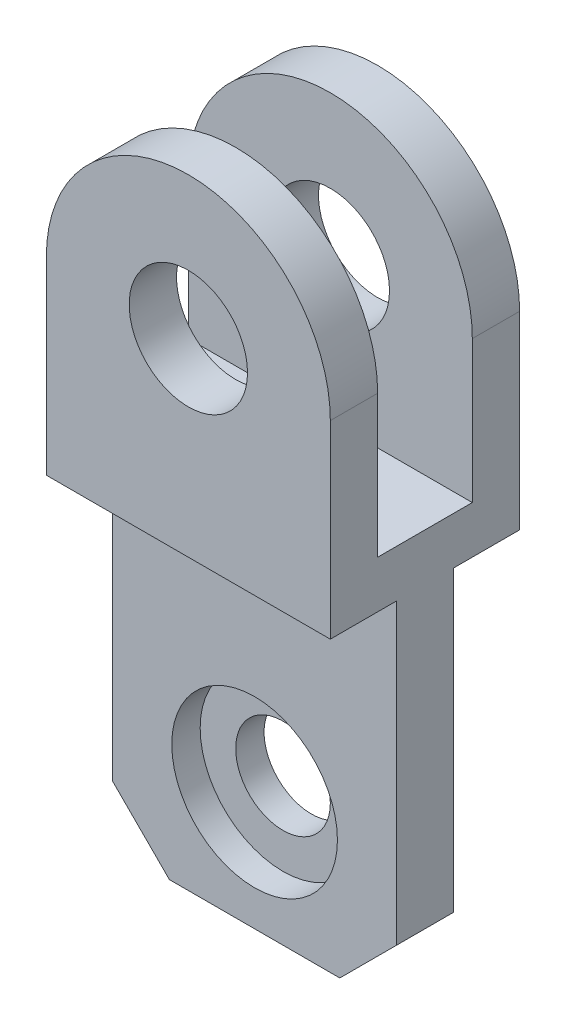
ISO-10303-21;
HEADER;
FILE_DESCRIPTION(('STEP AP214'),'2;1');
FILE_NAME('part.step','',(''),(''),'','','');
FILE_SCHEMA(('AUTOMOTIVE_DESIGN { 1 0 10303 214 1 1 1 1 }'));
ENDSEC;
DATA;
#1=APPLICATION_CONTEXT('core data for automotive mechanical design processes');
#2=APPLICATION_PROTOCOL_DEFINITION('international standard','automotive_design',2000,#1);
#3=PRODUCT_CONTEXT('',#1,'mechanical');
#4=PRODUCT('Part','Part','',(#3));
#5=PRODUCT_RELATED_PRODUCT_CATEGORY('part','',(#4));
#6=PRODUCT_DEFINITION_FORMATION('','',#4);
#7=PRODUCT_DEFINITION_CONTEXT('part definition',#1,'design');
#8=PRODUCT_DEFINITION('design','',#6,#7);
#9=PRODUCT_DEFINITION_SHAPE('','',#8);
#10=(LENGTH_UNIT() NAMED_UNIT(*) SI_UNIT(.MILLI.,.METRE.));
#11=(NAMED_UNIT(*) PLANE_ANGLE_UNIT() SI_UNIT($,.RADIAN.));
#12=(NAMED_UNIT(*) SI_UNIT($,.STERADIAN.) SOLID_ANGLE_UNIT());
#13=UNCERTAINTY_MEASURE_WITH_UNIT(LENGTH_MEASURE(1.E-05),#10,'distance_accuracy_value','');
#14=(GEOMETRIC_REPRESENTATION_CONTEXT(3) GLOBAL_UNCERTAINTY_ASSIGNED_CONTEXT((#13)) GLOBAL_UNIT_ASSIGNED_CONTEXT((#10,
#11,#12)) REPRESENTATION_CONTEXT('',''));
#15=CARTESIAN_POINT('',(0.,0.,0.));
#16=DIRECTION('',(0.,0.,1.));
#17=DIRECTION('',(1.,0.,0.));
#18=AXIS2_PLACEMENT_3D('',#15,#16,#17);
#19=CARTESIAN_POINT('',(-6.,0.,12.));
#20=DIRECTION('',(1.,0.,0.));
#21=DIRECTION('',(0.,0.,-1.));
#22=AXIS2_PLACEMENT_3D('',#19,#20,#21);
#23=PLANE('',#22);
#24=DIRECTION('',(0.,-1.,0.));
#25=VECTOR('',#24,1.);
#26=CARTESIAN_POINT('',(-6.,0.,0.));
#27=LINE('',#26,#25);
#28=CARTESIAN_POINT('',(-6.,0.,0.));
#29=VERTEX_POINT('',#28);
#30=CARTESIAN_POINT('',(-6.,-63.,0.));
#31=VERTEX_POINT('',#30);
#32=EDGE_CURVE('E126',#29,#31,#27,.T.);
#33=ORIENTED_EDGE('',*,*,#32,.T.);
#34=DIRECTION('',(0.,0.,-1.));
#35=VECTOR('',#34,1.);
#36=CARTESIAN_POINT('',(-6.,-63.,12.));
#37=LINE('',#36,#35);
#38=CARTESIAN_POINT('',(-6.,-63.,12.));
#39=VERTEX_POINT('',#38);
#40=EDGE_CURVE('E11',#39,#31,#37,.T.);
#41=ORIENTED_EDGE('',*,*,#40,.F.);
#42=DIRECTION('',(0.,-1.,0.));
#43=VECTOR('',#42,1.);
#44=CARTESIAN_POINT('',(-6.,0.,12.));
#45=LINE('',#44,#43);
#46=CARTESIAN_POINT('',(-6.,0.,12.));
#47=VERTEX_POINT('',#46);
#48=EDGE_CURVE('E107',#47,#39,#45,.T.);
#49=ORIENTED_EDGE('',*,*,#48,.F.);
#50=DIRECTION('',(0.,0.,1.));
#51=VECTOR('',#50,1.);
#52=CARTESIAN_POINT('',(-6.,0.,16.));
#53=LINE('',#52,#51);
#54=CARTESIAN_POINT('',(-6.,0.,26.));
#55=VERTEX_POINT('',#54);
#56=EDGE_CURVE('E91',#47,#55,#53,.T.);
#57=ORIENTED_EDGE('',*,*,#56,.T.);
#58=DIRECTION('',(0.,1.,0.));
#59=VECTOR('',#58,1.);
#60=CARTESIAN_POINT('',(-6.,0.,26.));
#61=LINE('',#60,#59);
#62=CARTESIAN_POINT('',(-6.,40.,26.));
#63=VERTEX_POINT('',#62);
#64=EDGE_CURVE('E235',#55,#63,#61,.T.);
#65=ORIENTED_EDGE('',*,*,#64,.T.);
#66=DIRECTION('',(0.,0.,-1.));
#67=VECTOR('',#66,1.);
#68=CARTESIAN_POINT('',(-6.,40.,26.));
#69=LINE('',#68,#67);
#70=CARTESIAN_POINT('',(-6.,40.,16.));
#71=VERTEX_POINT('',#70);
#72=EDGE_CURVE('E232',#63,#71,#69,.T.);
#73=ORIENTED_EDGE('',*,*,#72,.T.);
#74=DIRECTION('',(0.,1.,0.));
#75=VECTOR('',#74,1.);
#76=CARTESIAN_POINT('',(-6.,0.,16.));
#77=LINE('',#76,#75);
#78=CARTESIAN_POINT('',(-6.,10.,16.));
#79=VERTEX_POINT('',#78);
#80=EDGE_CURVE('E220',#79,#71,#77,.T.);
#81=ORIENTED_EDGE('',*,*,#80,.F.);
#82=DIRECTION('',(0.,0.,1.));
#83=VECTOR('',#82,1.);
#84=CARTESIAN_POINT('',(-6.,10.,16.));
#85=LINE('',#84,#83);
#86=CARTESIAN_POINT('',(-6.,10.,-4.));
#87=VERTEX_POINT('',#86);
#88=EDGE_CURVE('E270',#87,#79,#85,.T.);
#89=ORIENTED_EDGE('',*,*,#88,.F.);
#90=DIRECTION('',(0.,1.,0.));
#91=VECTOR('',#90,1.);
#92=CARTESIAN_POINT('',(-6.,0.,-4.));
#93=LINE('',#92,#91);
#94=CARTESIAN_POINT('',(-6.,40.,-4.));
#95=VERTEX_POINT('',#94);
#96=EDGE_CURVE('E242',#87,#95,#93,.T.);
#97=ORIENTED_EDGE('',*,*,#96,.T.);
#98=DIRECTION('',(0.,0.,-1.));
#99=VECTOR('',#98,1.);
#100=CARTESIAN_POINT('',(-6.,40.,-14.));
#101=LINE('',#100,#99);
#102=CARTESIAN_POINT('',(-6.,40.,-14.));
#103=VERTEX_POINT('',#102);
#104=EDGE_CURVE('E253',#95,#103,#101,.T.);
#105=ORIENTED_EDGE('',*,*,#104,.T.);
#106=DIRECTION('',(0.,-1.,0.));
#107=VECTOR('',#106,1.);
#108=CARTESIAN_POINT('',(-6.,0.,-14.));
#109=LINE('',#108,#107);
#110=CARTESIAN_POINT('',(-6.,0.,-14.));
#111=VERTEX_POINT('',#110);
#112=EDGE_CURVE('E258',#103,#111,#109,.T.);
#113=ORIENTED_EDGE('',*,*,#112,.T.);
#114=EDGE_CURVE('E277',#111,#29,#53,.T.);
#115=ORIENTED_EDGE('',*,*,#114,.T.);
#116=EDGE_LOOP('',(#33,#41,#49,#57,#65,#73,#81,#89,#97,#105,#113,#115));
#117=FACE_BOUND('',#116,.T.);
#118=ADVANCED_FACE('F44',(#117),#23,.F.);
#119=CARTESIAN_POINT('',(-6.,-63.,12.));
#120=DIRECTION('',(0.707106781186547,0.707106781186548,0.));
#121=DIRECTION('',(-0.707106781186548,0.707106781186547,0.));
#122=AXIS2_PLACEMENT_3D('',#119,#120,#121);
#123=PLANE('',#122);
#124=DIRECTION('',(0.707106781186548,-0.707106781186547,0.));
#125=VECTOR('',#124,1.);
#126=CARTESIAN_POINT('',(-6.,-63.,0.));
#127=LINE('',#126,#125);
#128=CARTESIAN_POINT('',(6.,-75.,0.));
#129=VERTEX_POINT('',#128);
#130=EDGE_CURVE('E114',#31,#129,#127,.T.);
#131=ORIENTED_EDGE('',*,*,#130,.T.);
#132=DIRECTION('',(0.,0.,-1.));
#133=VECTOR('',#132,1.);
#134=CARTESIAN_POINT('',(6.,-75.,12.));
#135=LINE('',#134,#133);
#136=CARTESIAN_POINT('',(6.,-75.,12.));
#137=VERTEX_POINT('',#136);
#138=EDGE_CURVE('E53',#137,#129,#135,.T.);
#139=ORIENTED_EDGE('',*,*,#138,.F.);
#140=DIRECTION('',(0.707106781186548,-0.707106781186547,0.));
#141=VECTOR('',#140,1.);
#142=CARTESIAN_POINT('',(-6.,-63.,12.));
#143=LINE('',#142,#141);
#144=EDGE_CURVE('E101',#39,#137,#143,.T.);
#145=ORIENTED_EDGE('',*,*,#144,.F.);
#146=ORIENTED_EDGE('',*,*,#40,.T.);
#147=EDGE_LOOP('',(#131,#139,#145,#146));
#148=FACE_BOUND('',#147,.T.);
#149=ADVANCED_FACE('F113',(#148),#123,.F.);
#150=CARTESIAN_POINT('',(6.,-75.,12.));
#151=DIRECTION('',(0.,1.,0.));
#152=DIRECTION('',(0.,0.,1.));
#153=AXIS2_PLACEMENT_3D('',#150,#151,#152);
#154=PLANE('',#153);
#155=DIRECTION('',(1.,0.,0.));
#156=VECTOR('',#155,1.);
#157=CARTESIAN_POINT('',(6.,-75.,0.));
#158=LINE('',#157,#156);
#159=CARTESIAN_POINT('',(42.,-75.,0.));
#160=VERTEX_POINT('',#159);
#161=EDGE_CURVE('E78',#129,#160,#158,.T.);
#162=ORIENTED_EDGE('',*,*,#161,.T.);
#163=DIRECTION('',(0.,0.,-1.));
#164=VECTOR('',#163,1.);
#165=CARTESIAN_POINT('',(42.,-75.,12.));
#166=LINE('',#165,#164);
#167=CARTESIAN_POINT('',(42.,-75.,12.));
#168=VERTEX_POINT('',#167);
#169=EDGE_CURVE('E116',#168,#160,#166,.T.);
#170=ORIENTED_EDGE('',*,*,#169,.F.);
#171=DIRECTION('',(1.,0.,0.));
#172=VECTOR('',#171,1.);
#173=CARTESIAN_POINT('',(6.,-75.,12.));
#174=LINE('',#173,#172);
#175=EDGE_CURVE('E108',#137,#168,#174,.T.);
#176=ORIENTED_EDGE('',*,*,#175,.F.);
#177=ORIENTED_EDGE('',*,*,#138,.T.);
#178=EDGE_LOOP('',(#162,#170,#176,#177));
#179=FACE_BOUND('',#178,.T.);
#180=ADVANCED_FACE('F117',(#179),#154,.F.);
#181=CARTESIAN_POINT('',(54.,-63.,12.));
#182=DIRECTION('',(-0.707106781186547,0.707106781186548,0.));
#183=DIRECTION('',(-0.707106781186548,-0.707106781186547,0.));
#184=AXIS2_PLACEMENT_3D('',#181,#182,#183);
#185=PLANE('',#184);
#186=DIRECTION('',(0.707106781186548,0.707106781186547,0.));
#187=VECTOR('',#186,1.);
#188=CARTESIAN_POINT('',(54.,-63.,0.));
#189=LINE('',#188,#187);
#190=CARTESIAN_POINT('',(54.,-63.,0.));
#191=VERTEX_POINT('',#190);
#192=EDGE_CURVE('E87',#160,#191,#189,.T.);
#193=ORIENTED_EDGE('',*,*,#192,.T.);
#194=DIRECTION('',(0.,0.,-1.));
#195=VECTOR('',#194,1.);
#196=CARTESIAN_POINT('',(54.,-63.,12.));
#197=LINE('',#196,#195);
#198=CARTESIAN_POINT('',(54.,-63.,12.));
#199=VERTEX_POINT('',#198);
#200=EDGE_CURVE('E123',#199,#191,#197,.T.);
#201=ORIENTED_EDGE('',*,*,#200,.F.);
#202=DIRECTION('',(0.707106781186548,0.707106781186547,0.));
#203=VECTOR('',#202,1.);
#204=CARTESIAN_POINT('',(54.,-63.,12.));
#205=LINE('',#204,#203);
#206=EDGE_CURVE('E65',#168,#199,#205,.T.);
#207=ORIENTED_EDGE('',*,*,#206,.F.);
#208=ORIENTED_EDGE('',*,*,#169,.T.);
#209=EDGE_LOOP('',(#193,#201,#207,#208));
#210=FACE_BOUND('',#209,.T.);
#211=ADVANCED_FACE('F136',(#210),#185,.F.);
#212=CARTESIAN_POINT('',(54.,-63.,12.));
#213=DIRECTION('',(-1.,0.,0.));
#214=DIRECTION('',(0.,0.,1.));
#215=AXIS2_PLACEMENT_3D('',#212,#213,#214);
#216=PLANE('',#215);
#217=DIRECTION('',(0.,1.,0.));
#218=VECTOR('',#217,1.);
#219=CARTESIAN_POINT('',(54.,-63.,0.));
#220=LINE('',#219,#218);
#221=CARTESIAN_POINT('',(54.,0.,0.));
#222=VERTEX_POINT('',#221);
#223=EDGE_CURVE('E133',#191,#222,#220,.T.);
#224=ORIENTED_EDGE('',*,*,#223,.T.);
#225=DIRECTION('',(0.,0.,-1.));
#226=VECTOR('',#225,1.);
#227=CARTESIAN_POINT('',(54.,0.,-4.));
#228=LINE('',#227,#226);
#229=CARTESIAN_POINT('',(54.,0.,-14.));
#230=VERTEX_POINT('',#229);
#231=EDGE_CURVE('E154',#222,#230,#228,.T.);
#232=ORIENTED_EDGE('',*,*,#231,.T.);
#233=DIRECTION('',(0.,-1.,0.));
#234=VECTOR('',#233,1.);
#235=CARTESIAN_POINT('',(54.,0.,-14.));
#236=LINE('',#235,#234);
#237=CARTESIAN_POINT('',(54.,40.,-14.));
#238=VERTEX_POINT('',#237);
#239=EDGE_CURVE('E257',#238,#230,#236,.T.);
#240=ORIENTED_EDGE('',*,*,#239,.F.);
#241=DIRECTION('',(0.,0.,-1.));
#242=VECTOR('',#241,1.);
#243=CARTESIAN_POINT('',(54.,40.,-4.));
#244=LINE('',#243,#242);
#245=CARTESIAN_POINT('',(54.,40.,-4.));
#246=VERTEX_POINT('',#245);
#247=EDGE_CURVE('E252',#246,#238,#244,.T.);
#248=ORIENTED_EDGE('',*,*,#247,.F.);
#249=DIRECTION('',(0.,1.,0.));
#250=VECTOR('',#249,1.);
#251=CARTESIAN_POINT('',(54.,0.,-4.));
#252=LINE('',#251,#250);
#253=CARTESIAN_POINT('',(54.,10.,-4.));
#254=VERTEX_POINT('',#253);
#255=EDGE_CURVE('E243',#254,#246,#252,.T.);
#256=ORIENTED_EDGE('',*,*,#255,.F.);
#257=DIRECTION('',(0.,0.,-1.));
#258=VECTOR('',#257,1.);
#259=CARTESIAN_POINT('',(54.,10.,-4.));
#260=LINE('',#259,#258);
#261=CARTESIAN_POINT('',(54.,10.,16.));
#262=VERTEX_POINT('',#261);
#263=EDGE_CURVE('E214',#262,#254,#260,.T.);
#264=ORIENTED_EDGE('',*,*,#263,.F.);
#265=DIRECTION('',(0.,1.,0.));
#266=VECTOR('',#265,1.);
#267=CARTESIAN_POINT('',(54.,0.,16.));
#268=LINE('',#267,#266);
#269=CARTESIAN_POINT('',(54.,40.,16.));
#270=VERTEX_POINT('',#269);
#271=EDGE_CURVE('E210',#262,#270,#268,.T.);
#272=ORIENTED_EDGE('',*,*,#271,.T.);
#273=DIRECTION('',(0.,0.,-1.));
#274=VECTOR('',#273,1.);
#275=CARTESIAN_POINT('',(54.,40.,26.));
#276=LINE('',#275,#274);
#277=CARTESIAN_POINT('',(54.,40.,26.));
#278=VERTEX_POINT('',#277);
#279=EDGE_CURVE('E208',#278,#270,#276,.T.);
#280=ORIENTED_EDGE('',*,*,#279,.F.);
#281=DIRECTION('',(0.,1.,0.));
#282=VECTOR('',#281,1.);
#283=CARTESIAN_POINT('',(54.,0.,26.));
#284=LINE('',#283,#282);
#285=CARTESIAN_POINT('',(54.,0.,26.));
#286=VERTEX_POINT('',#285);
#287=EDGE_CURVE('E226',#286,#278,#284,.T.);
#288=ORIENTED_EDGE('',*,*,#287,.F.);
#289=CARTESIAN_POINT('',(54.,0.,12.));
#290=VERTEX_POINT('',#289);
#291=EDGE_CURVE('E272',#286,#290,#228,.T.);
#292=ORIENTED_EDGE('',*,*,#291,.T.);
#293=DIRECTION('',(0.,1.,0.));
#294=VECTOR('',#293,1.);
#295=CARTESIAN_POINT('',(54.,-63.,12.));
#296=LINE('',#295,#294);
#297=EDGE_CURVE('E119',#199,#290,#296,.T.);
#298=ORIENTED_EDGE('',*,*,#297,.F.);
#299=ORIENTED_EDGE('',*,*,#200,.T.);
#300=EDGE_LOOP('',(#224,#232,#240,#248,#256,#264,#272,#280,#288,#292,#298,#299));
#301=FACE_BOUND('',#300,.T.);
#302=ADVANCED_FACE('F149',(#301),#216,.F.);
#303=CARTESIAN_POINT('',(0.,0.,12.));
#304=DIRECTION('',(0.,0.,1.));
#305=DIRECTION('',(1.,0.,0.));
#306=AXIS2_PLACEMENT_3D('',#303,#304,#305);
#307=PLANE('',#306);
#308=CARTESIAN_POINT('',(24.,-50.,12.));
#309=DIRECTION('',(0.,0.,1.));
#310=DIRECTION('',(1.,0.,0.));
#311=AXIS2_PLACEMENT_3D('',#308,#309,#310);
#312=CIRCLE('',#311,17.5);
#313=CARTESIAN_POINT('',(41.5,-50.,12.));
#314=VERTEX_POINT('',#313);
#315=EDGE_CURVE('E313',#314,#314,#312,.T.);
#316=ORIENTED_EDGE('',*,*,#315,.F.);
#317=EDGE_LOOP('',(#316));
#318=FACE_BOUND('',#317,.T.);
#319=DIRECTION('',(-1.,0.,0.));
#320=VECTOR('',#319,1.);
#321=CARTESIAN_POINT('',(-6.,0.,12.));
#322=LINE('',#321,#320);
#323=EDGE_CURVE('E138',#290,#47,#322,.T.);
#324=ORIENTED_EDGE('',*,*,#323,.T.);
#325=ORIENTED_EDGE('',*,*,#48,.T.);
#326=ORIENTED_EDGE('',*,*,#144,.T.);
#327=ORIENTED_EDGE('',*,*,#175,.T.);
#328=ORIENTED_EDGE('',*,*,#206,.T.);
#329=ORIENTED_EDGE('',*,*,#297,.T.);
#330=EDGE_LOOP('',(#324,#325,#326,#327,#328,#329));
#331=FACE_BOUND('',#330,.T.);
#332=ADVANCED_FACE('F106',(#318,#331),#307,.T.);
#333=CARTESIAN_POINT('',(0.,0.,0.));
#334=DIRECTION('',(0.,0.,1.));
#335=DIRECTION('',(1.,0.,0.));
#336=AXIS2_PLACEMENT_3D('',#333,#334,#335);
#337=PLANE('',#336);
#338=CARTESIAN_POINT('',(24.,-50.,0.));
#339=DIRECTION('',(0.,0.,1.));
#340=DIRECTION('',(1.,0.,0.));
#341=AXIS2_PLACEMENT_3D('',#338,#339,#340);
#342=CIRCLE('',#341,10.);
#343=CARTESIAN_POINT('',(34.,-50.,0.));
#344=VERTEX_POINT('',#343);
#345=EDGE_CURVE('E320',#344,#344,#342,.T.);
#346=ORIENTED_EDGE('',*,*,#345,.T.);
#347=EDGE_LOOP('',(#346));
#348=FACE_BOUND('',#347,.T.);
#349=DIRECTION('',(-1.,0.,0.));
#350=VECTOR('',#349,1.);
#351=CARTESIAN_POINT('',(-6.,0.,0.));
#352=LINE('',#351,#350);
#353=EDGE_CURVE('E127',#222,#29,#352,.T.);
#354=ORIENTED_EDGE('',*,*,#353,.F.);
#355=ORIENTED_EDGE('',*,*,#223,.F.);
#356=ORIENTED_EDGE('',*,*,#192,.F.);
#357=ORIENTED_EDGE('',*,*,#161,.F.);
#358=ORIENTED_EDGE('',*,*,#130,.F.);
#359=ORIENTED_EDGE('',*,*,#32,.F.);
#360=EDGE_LOOP('',(#354,#355,#356,#357,#358,#359));
#361=FACE_BOUND('',#360,.T.);
#362=ADVANCED_FACE('F144',(#348,#361),#337,.F.);
#363=CARTESIAN_POINT('',(0.,0.,0.));
#364=DIRECTION('',(0.,-1.,0.));
#365=DIRECTION('',(0.,0.,-1.));
#366=AXIS2_PLACEMENT_3D('',#363,#364,#365);
#367=PLANE('',#366);
#368=ORIENTED_EDGE('',*,*,#323,.F.);
#369=ORIENTED_EDGE('',*,*,#291,.F.);
#370=DIRECTION('',(-1.,0.,0.));
#371=VECTOR('',#370,1.);
#372=CARTESIAN_POINT('',(54.,0.,26.));
#373=LINE('',#372,#371);
#374=EDGE_CURVE('E227',#286,#55,#373,.T.);
#375=ORIENTED_EDGE('',*,*,#374,.T.);
#376=ORIENTED_EDGE('',*,*,#56,.F.);
#377=EDGE_LOOP('',(#368,#369,#375,#376));
#378=FACE_BOUND('',#377,.T.);
#379=ADVANCED_FACE('F282',(#378),#367,.T.);
#380=CARTESIAN_POINT('',(0.,10.,0.));
#381=DIRECTION('',(0.,-1.,0.));
#382=DIRECTION('',(0.,0.,-1.));
#383=AXIS2_PLACEMENT_3D('',#380,#381,#382);
#384=PLANE('',#383);
#385=ORIENTED_EDGE('',*,*,#88,.T.);
#386=DIRECTION('',(1.,0.,0.));
#387=VECTOR('',#386,1.);
#388=CARTESIAN_POINT('',(54.,10.,16.));
#389=LINE('',#388,#387);
#390=EDGE_CURVE('E266',#79,#262,#389,.T.);
#391=ORIENTED_EDGE('',*,*,#390,.T.);
#392=ORIENTED_EDGE('',*,*,#263,.T.);
#393=DIRECTION('',(-1.,0.,0.));
#394=VECTOR('',#393,1.);
#395=CARTESIAN_POINT('',(-6.,10.,-4.));
#396=LINE('',#395,#394);
#397=EDGE_CURVE('E128',#254,#87,#396,.T.);
#398=ORIENTED_EDGE('',*,*,#397,.T.);
#399=EDGE_LOOP('',(#385,#391,#392,#398));
#400=FACE_BOUND('',#399,.T.);
#401=ADVANCED_FACE('F299',(#400),#384,.F.);
#402=ORIENTED_EDGE('',*,*,#231,.F.);
#403=ORIENTED_EDGE('',*,*,#353,.T.);
#404=ORIENTED_EDGE('',*,*,#114,.F.);
#405=DIRECTION('',(-1.,0.,0.));
#406=VECTOR('',#405,1.);
#407=CARTESIAN_POINT('',(54.,0.,-14.));
#408=LINE('',#407,#406);
#409=EDGE_CURVE('E256',#230,#111,#408,.T.);
#410=ORIENTED_EDGE('',*,*,#409,.F.);
#411=EDGE_LOOP('',(#402,#403,#404,#410));
#412=FACE_BOUND('',#411,.T.);
#413=ADVANCED_FACE('F290',(#412),#367,.T.);
#414=CARTESIAN_POINT('',(54.,0.,-14.));
#415=DIRECTION('',(0.,0.,-1.));
#416=DIRECTION('',(-1.,0.,0.));
#417=AXIS2_PLACEMENT_3D('',#414,#415,#416);
#418=PLANE('',#417);
#419=CARTESIAN_POINT('',(24.,40.,-14.));
#420=DIRECTION('',(0.,0.,1.));
#421=DIRECTION('',(1.,0.,0.));
#422=AXIS2_PLACEMENT_3D('',#419,#420,#421);
#423=CIRCLE('',#422,12.5);
#424=CARTESIAN_POINT('',(36.5,40.,-14.));
#425=VERTEX_POINT('',#424);
#426=EDGE_CURVE('E306',#425,#425,#423,.T.);
#427=ORIENTED_EDGE('',*,*,#426,.T.);
#428=EDGE_LOOP('',(#427));
#429=FACE_BOUND('',#428,.T.);
#430=ORIENTED_EDGE('',*,*,#112,.F.);
#431=CARTESIAN_POINT('',(24.,40.,-14.));
#432=DIRECTION('',(0.,0.,-1.));
#433=DIRECTION('',(-1.,0.,0.));
#434=AXIS2_PLACEMENT_3D('',#431,#432,#433);
#435=CIRCLE('',#434,30.);
#436=EDGE_CURVE('E246',#103,#238,#435,.T.);
#437=ORIENTED_EDGE('',*,*,#436,.T.);
#438=ORIENTED_EDGE('',*,*,#239,.T.);
#439=ORIENTED_EDGE('',*,*,#409,.T.);
#440=EDGE_LOOP('',(#430,#437,#438,#439));
#441=FACE_BOUND('',#440,.T.);
#442=ADVANCED_FACE('F289',(#429,#441),#418,.T.);
#443=CARTESIAN_POINT('',(24.,40.,-4.));
#444=DIRECTION('',(0.,0.,-1.));
#445=DIRECTION('',(-1.,0.,0.));
#446=AXIS2_PLACEMENT_3D('',#443,#444,#445);
#447=CYLINDRICAL_SURFACE('',#446,30.);
#448=CARTESIAN_POINT('',(24.,40.,-4.));
#449=DIRECTION('',(0.,0.,-1.));
#450=DIRECTION('',(-1.,0.,0.));
#451=AXIS2_PLACEMENT_3D('',#448,#449,#450);
#452=CIRCLE('',#451,30.);
#453=EDGE_CURVE('E247',#95,#246,#452,.T.);
#454=ORIENTED_EDGE('',*,*,#453,.T.);
#455=ORIENTED_EDGE('',*,*,#247,.T.);
#456=ORIENTED_EDGE('',*,*,#436,.F.);
#457=ORIENTED_EDGE('',*,*,#104,.F.);
#458=EDGE_LOOP('',(#454,#455,#456,#457));
#459=FACE_BOUND('',#458,.T.);
#460=ADVANCED_FACE('F292',(#459),#447,.T.);
#461=CARTESIAN_POINT('',(24.,40.,-4.));
#462=DIRECTION('',(0.,0.,-1.));
#463=DIRECTION('',(-1.,0.,0.));
#464=AXIS2_PLACEMENT_3D('',#461,#462,#463);
#465=PLANE('',#464);
#466=CARTESIAN_POINT('',(24.,40.,-4.));
#467=DIRECTION('',(0.,0.,-1.));
#468=DIRECTION('',(-1.,0.,0.));
#469=AXIS2_PLACEMENT_3D('',#466,#467,#468);
#470=CIRCLE('',#469,12.5);
#471=CARTESIAN_POINT('',(11.5,40.,-4.));
#472=VERTEX_POINT('',#471);
#473=EDGE_CURVE('E297',#472,#472,#470,.T.);
#474=ORIENTED_EDGE('',*,*,#473,.T.);
#475=EDGE_LOOP('',(#474));
#476=FACE_BOUND('',#475,.T.);
#477=ORIENTED_EDGE('',*,*,#397,.F.);
#478=ORIENTED_EDGE('',*,*,#255,.T.);
#479=ORIENTED_EDGE('',*,*,#453,.F.);
#480=ORIENTED_EDGE('',*,*,#96,.F.);
#481=EDGE_LOOP('',(#477,#478,#479,#480));
#482=FACE_BOUND('',#481,.T.);
#483=ADVANCED_FACE('F298',(#476,#482),#465,.F.);
#484=CARTESIAN_POINT('',(54.,0.,26.));
#485=DIRECTION('',(0.,0.,1.));
#486=DIRECTION('',(1.,0.,0.));
#487=AXIS2_PLACEMENT_3D('',#484,#485,#486);
#488=PLANE('',#487);
#489=CARTESIAN_POINT('',(24.,40.,26.));
#490=DIRECTION('',(0.,0.,1.));
#491=DIRECTION('',(1.,0.,0.));
#492=AXIS2_PLACEMENT_3D('',#489,#490,#491);
#493=CIRCLE('',#492,12.5);
#494=CARTESIAN_POINT('',(36.5,40.,26.));
#495=VERTEX_POINT('',#494);
#496=EDGE_CURVE('E308',#495,#495,#493,.T.);
#497=ORIENTED_EDGE('',*,*,#496,.F.);
#498=EDGE_LOOP('',(#497));
#499=FACE_BOUND('',#498,.T.);
#500=ORIENTED_EDGE('',*,*,#287,.T.);
#501=CARTESIAN_POINT('',(24.,40.,26.));
#502=DIRECTION('',(0.,0.,1.));
#503=DIRECTION('',(1.,0.,0.));
#504=AXIS2_PLACEMENT_3D('',#501,#502,#503);
#505=CIRCLE('',#504,30.);
#506=EDGE_CURVE('E219',#278,#63,#505,.T.);
#507=ORIENTED_EDGE('',*,*,#506,.T.);
#508=ORIENTED_EDGE('',*,*,#64,.F.);
#509=ORIENTED_EDGE('',*,*,#374,.F.);
#510=EDGE_LOOP('',(#500,#507,#508,#509));
#511=FACE_BOUND('',#510,.T.);
#512=ADVANCED_FACE('F281',(#499,#511),#488,.T.);
#513=CARTESIAN_POINT('',(24.,40.,16.));
#514=DIRECTION('',(0.,0.,1.));
#515=DIRECTION('',(1.,0.,0.));
#516=AXIS2_PLACEMENT_3D('',#513,#514,#515);
#517=CYLINDRICAL_SURFACE('',#516,30.);
#518=ORIENTED_EDGE('',*,*,#279,.T.);
#519=CARTESIAN_POINT('',(24.,40.,16.));
#520=DIRECTION('',(0.,0.,1.));
#521=DIRECTION('',(1.,0.,0.));
#522=AXIS2_PLACEMENT_3D('',#519,#520,#521);
#523=CIRCLE('',#522,30.);
#524=EDGE_CURVE('E223',#270,#71,#523,.T.);
#525=ORIENTED_EDGE('',*,*,#524,.T.);
#526=ORIENTED_EDGE('',*,*,#72,.F.);
#527=ORIENTED_EDGE('',*,*,#506,.F.);
#528=EDGE_LOOP('',(#518,#525,#526,#527));
#529=FACE_BOUND('',#528,.T.);
#530=ADVANCED_FACE('F225',(#529),#517,.T.);
#531=CARTESIAN_POINT('',(24.,40.,16.));
#532=DIRECTION('',(0.,0.,1.));
#533=DIRECTION('',(1.,0.,0.));
#534=AXIS2_PLACEMENT_3D('',#531,#532,#533);
#535=PLANE('',#534);
#536=CARTESIAN_POINT('',(24.,40.,16.));
#537=DIRECTION('',(0.,0.,1.));
#538=DIRECTION('',(1.,0.,0.));
#539=AXIS2_PLACEMENT_3D('',#536,#537,#538);
#540=CIRCLE('',#539,12.5);
#541=CARTESIAN_POINT('',(36.5,40.,16.));
#542=VERTEX_POINT('',#541);
#543=EDGE_CURVE('E48',#542,#542,#540,.T.);
#544=ORIENTED_EDGE('',*,*,#543,.T.);
#545=EDGE_LOOP('',(#544));
#546=FACE_BOUND('',#545,.T.);
#547=ORIENTED_EDGE('',*,*,#390,.F.);
#548=ORIENTED_EDGE('',*,*,#80,.T.);
#549=ORIENTED_EDGE('',*,*,#524,.F.);
#550=ORIENTED_EDGE('',*,*,#271,.F.);
#551=EDGE_LOOP('',(#547,#548,#549,#550));
#552=FACE_BOUND('',#551,.T.);
#553=ADVANCED_FACE('F229',(#546,#552),#535,.F.);
#554=CARTESIAN_POINT('',(24.,40.,-14.));
#555=DIRECTION('',(0.,0.,1.));
#556=DIRECTION('',(1.,0.,0.));
#557=AXIS2_PLACEMENT_3D('',#554,#555,#556);
#558=CYLINDRICAL_SURFACE('',#557,12.5);
#559=ORIENTED_EDGE('',*,*,#496,.T.);
#560=EDGE_LOOP('',(#559));
#561=FACE_BOUND('',#560,.T.);
#562=ORIENTED_EDGE('',*,*,#543,.F.);
#563=EDGE_LOOP('',(#562));
#564=FACE_BOUND('',#563,.T.);
#565=ADVANCED_FACE('F439',(#561,#564),#558,.F.);
#566=ORIENTED_EDGE('',*,*,#426,.F.);
#567=EDGE_LOOP('',(#566));
#568=FACE_BOUND('',#567,.T.);
#569=ORIENTED_EDGE('',*,*,#473,.F.);
#570=EDGE_LOOP('',(#569));
#571=FACE_BOUND('',#570,.T.);
#572=ADVANCED_FACE('F345',(#568,#571),#558,.F.);
#573=CARTESIAN_POINT('',(24.,-50.,6.));
#574=DIRECTION('',(0.,0.,1.));
#575=DIRECTION('',(1.,0.,0.));
#576=AXIS2_PLACEMENT_3D('',#573,#574,#575);
#577=CYLINDRICAL_SURFACE('',#576,17.5);
#578=CARTESIAN_POINT('',(24.,-50.,6.));
#579=DIRECTION('',(0.,0.,1.));
#580=DIRECTION('',(1.,0.,0.));
#581=AXIS2_PLACEMENT_3D('',#578,#579,#580);
#582=CIRCLE('',#581,17.5);
#583=CARTESIAN_POINT('',(41.5,-50.,6.));
#584=VERTEX_POINT('',#583);
#585=EDGE_CURVE('E311',#584,#584,#582,.T.);
#586=ORIENTED_EDGE('',*,*,#585,.F.);
#587=EDGE_LOOP('',(#586));
#588=FACE_BOUND('',#587,.T.);
#589=ORIENTED_EDGE('',*,*,#315,.T.);
#590=EDGE_LOOP('',(#589));
#591=FACE_BOUND('',#590,.T.);
#592=ADVANCED_FACE('F337',(#588,#591),#577,.F.);
#593=CARTESIAN_POINT('',(24.,-50.,6.));
#594=DIRECTION('',(0.,0.,1.));
#595=DIRECTION('',(1.,0.,0.));
#596=AXIS2_PLACEMENT_3D('',#593,#594,#595);
#597=PLANE('',#596);
#598=CARTESIAN_POINT('',(24.,-50.,6.));
#599=DIRECTION('',(0.,0.,1.));
#600=DIRECTION('',(1.,0.,0.));
#601=AXIS2_PLACEMENT_3D('',#598,#599,#600);
#602=CIRCLE('',#601,10.);
#603=CARTESIAN_POINT('',(34.,-50.,6.));
#604=VERTEX_POINT('',#603);
#605=EDGE_CURVE('E318',#604,#604,#602,.T.);
#606=ORIENTED_EDGE('',*,*,#605,.F.);
#607=EDGE_LOOP('',(#606));
#608=FACE_BOUND('',#607,.T.);
#609=ORIENTED_EDGE('',*,*,#585,.T.);
#610=EDGE_LOOP('',(#609));
#611=FACE_BOUND('',#610,.T.);
#612=ADVANCED_FACE('F328',(#608,#611),#597,.T.);
#613=CARTESIAN_POINT('',(24.,-50.,0.));
#614=DIRECTION('',(0.,0.,1.));
#615=DIRECTION('',(1.,0.,0.));
#616=AXIS2_PLACEMENT_3D('',#613,#614,#615);
#617=CYLINDRICAL_SURFACE('',#616,10.);
#618=ORIENTED_EDGE('',*,*,#345,.F.);
#619=EDGE_LOOP('',(#618));
#620=FACE_BOUND('',#619,.T.);
#621=ORIENTED_EDGE('',*,*,#605,.T.);
#622=EDGE_LOOP('',(#621));
#623=FACE_BOUND('',#622,.T.);
#624=ADVANCED_FACE('F329',(#620,#623),#617,.F.);
#625=CLOSED_SHELL('',(#118,#149,#180,#211,#302,#332,#362,#379,#401,#413,#442,#460,#483,#512,
#530,#553,#565,#572,#592,#612,#624));
#626=MANIFOLD_SOLID_BREP('B2',#625);
#627=ADVANCED_BREP_SHAPE_REPRESENTATION('',(#18,#626),#14);
#628=SHAPE_DEFINITION_REPRESENTATION(#9,#627);
ENDSEC;
END-ISO-10303-21;
